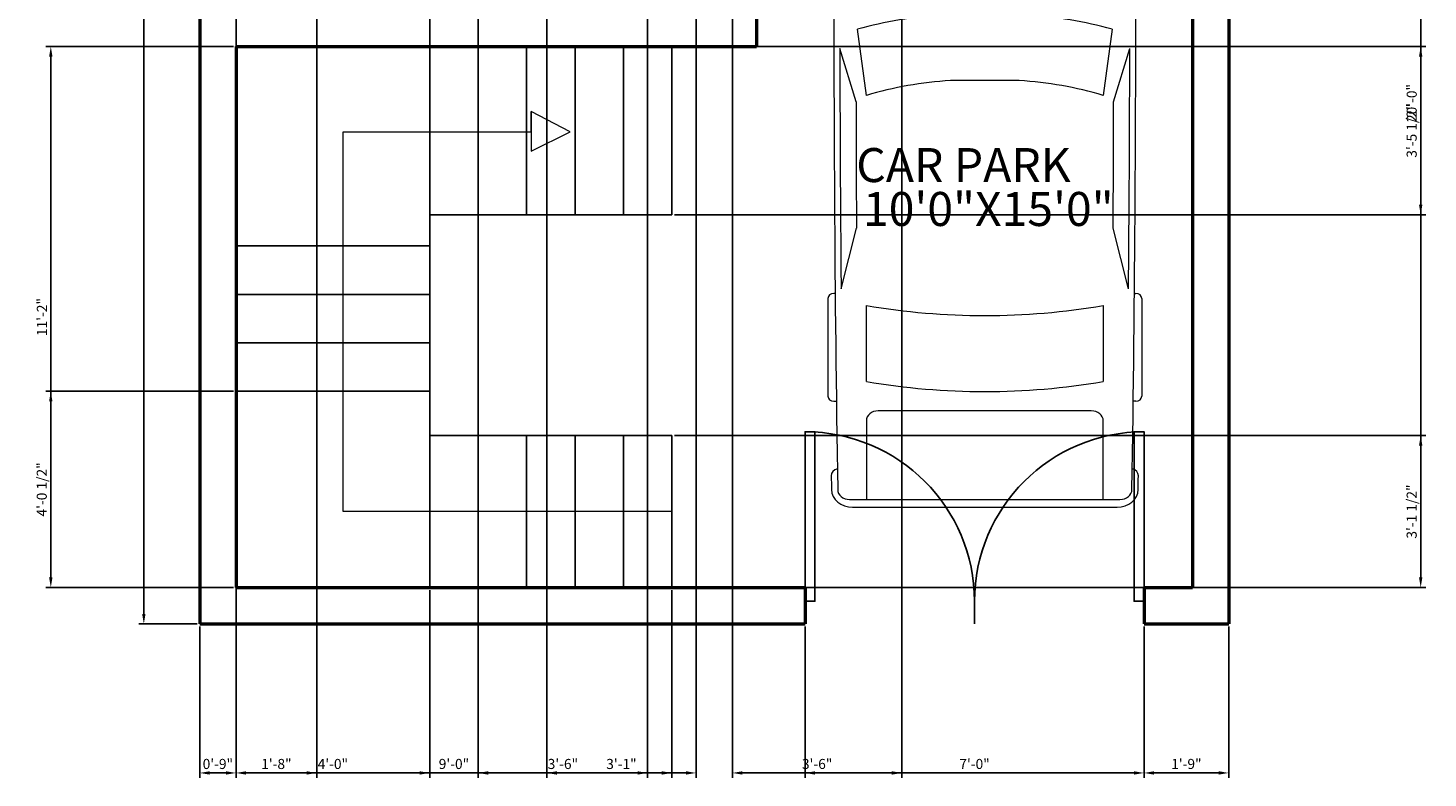
# Model space of a CAD drawing. Units: inches. Extents: x 758743 to 759108, y 3712801 to 3713581.
# Tile 1 of 4: x 758743 to 759090, y 3712801 to 3712987. Entities that reach past the tile are written whole.
import ezdxf

# ---------------------------------------------------------------- set-up
doc = ezdxf.new("R2010")
doc.units = ezdxf.units.IN
for name, color, linetype, lineweight in [('A-ANNO-DIMS', 2, 'Continuous', 18), ('A-ANNO-SYMB', 6, 'Continuous', 18), ('A-AREA-IDEN', 3, 'Continuous', 18), ('A-SITE-VEHI', 8, 'Continuous', 13), ('DOOR', 4, 'Continuous', 25), ('STAIRCASE', 6, 'Continuous', 25), ('WALL', 7, 'Continuous', 50)]:
    doc.layers.add(name, color=color, linetype=linetype, lineweight=lineweight)
doc.styles.get("Standard").update_dxf_attribs({"font": 'arial.ttf'})
doc.dimstyles.new('ISO-25', dxfattribs={"dimtxt": 2.5, "dimasz": 2.5, "dimexe": 1.25, "dimexo": 0.625, "dimtad": 1, "dimdec": 0, "dimlunit": 3, "dimtxsty": 'Standard', "dimcen": 2.5, "dimadec": 0, "dimazin": 0, "dimtfac": 1, "dimtdec": 0, "dimtmove": 0, "dimatfit": 3, "dimfxl": 1, "dimarcsym": 0})

# ---------------------------------------------------------------- blocks, each defined once
blk = doc.blocks.new('*U2')
for p, q in [((0, 0), (0, -100)), ((750, 0), (750, -100))]:
    blk.add_line(p, q)
blk.add_lwpolyline([(0, 0), (0, 750), (43.75, 750), (43.75, 0)], close=True)
blk.add_arc((0, 0), 750, 0, 90)
blk = doc.blocks.new('*U10')
for p, q in [((46.55, 38.89), (22.35, 38.89)), ((136.7, 38.89), (160.9, 38.89)), ((21.1, 37.41), (21.1, 36.83)), ((47.8, 37.39), (47.8, 37.41)), ((87.99, 31.87), (74.76, 35.92)), ((134.31, 35.6), (119.29, 31.78)), ((135.45, 37.07), (135.45, 37.41)), ((162.15, 37.41), (162.15, 36.77)), ((70.03, 31.54), (86.41, 29.35)), ((186.47, -33.5), (186.47, 33.5)), ((188.4, -32.76), (188.4, 32.76)), ((138.42, 29.35), (157.25, 29.35)), ((186.47, 29.35), (167.01, 29.35)), ((164.52, 26.39), (164.52, -26.39)), ((32.27, 11.63), (36.13, 17.17)), ((36.13, 17.17), (50.94, 17.17)), ((32.12, 9.51), (32.12, 11.15)), ((58.92, -10.77), (58.92, 10.77)), ((66.55, -10.53), (66.55, 10.53)), ((186.47, -10.53), (186.47, 10.53)), ((29.77, 9.51), (51.68, 9.51)), ((82.74, 8.5), (82.74, -8.5)), ((3.27, 6.13), (0.1, 0.41)), ((0, 0), (51.68, 0)), ((0.1, -0.41), (3.27, -6.13)), ((29.77, -9.51), (51.68, -9.51)), ((32.12, -9.51), (32.12, -11.15)), ((32.27, -11.63), (36.13, -17.17)), ((36.13, -17.17), (50.94, -17.17)), ((86.41, -29.35), (70.03, -31.54)), ((157.25, -29.35), (138.42, -29.35)), ((167.01, -29.35), (186.47, -29.35)), ((87.99, -31.87), (74.76, -35.92)), ((134.31, -35.6), (119.29, -31.78)), ((21.1, -37.41), (21.1, -36.83)), ((47.8, -37.39), (47.8, -37.41)), ((135.45, -37.07), (135.45, -37.41)), ((162.15, -37.41), (162.15, -36.77)), ((46.55, -38.89), (22.35, -38.89)), ((136.7, -38.89), (160.9, -38.89))]:
    blk.add_line(p, q)
for centre, major_axis, ratio, start_param, end_param in [((22.35, 37.41), (0, -1.48), 0.842304, 3.141593, 4.712389), ((46.55, 37.41), (0, 1.48), 0.842304, -1.570796, 0), ((136.7, 37.41), (0, -1.48), 0.842304, 3.141593, 4.712389), ((160.9, 37.41), (0, 1.48), 0.842304, -1.570796, 0), ((266.03, -27.52), (0, 313.31), 0.842304, 1.367076, 1.39176), ((41.19, -490.86), (0, 528.23), 0.842304, 0.00281, 0.075598), ((64.48, -10555.62), (0, 10593.03), 0.842304, -0.013397, 0.002797), ((64.48, -10555.62), (0, -10591.55), 0.842304, 3.133765, 3.140441), ((180.63, 35.84), (0, 2.22), 0.842304, -0.013017, 1.249894), ((64.48, -10556.36), (0, 10595.31), 0.842304, -0.013397, -0.013017), ((183.98, 33.5), (0, -2.96), 0.842304, 1.570796, 3.128196), ((183.98, 32.76), (0, -5.25), 0.842304, 1.570796, 3.128196), ((135.29, 5.39), (0, 81.77), 0.842304, 1.245306, 1.50788), ((95.79, -3666.35), (0, -3698.24), 0.842304, 3.134049, 3.144098), ((259.18, -27.52), (0, -305.3), 0.842304, 4.528606, 4.561838), ((37.47, -593.96), (0, -623.33), 0.842304, 3.096046, 3.200911), ((134.4, 5.39), (0, -89.78), 0.842304, 4.449482, 4.652344), ((149.6, 2.8), (0, -79.58), 0.842304, 4.372215, 4.640744), ((17.08, 0), (0, 147.02), 0.842304, 4.511394, 4.913384), ((35.91, 0), (0, 147.02), 0.842304, 4.511394, 4.913384), ((167.01, 26.39), (0, 2.96), 0.842304, 0, 1.570796), ((-204.49, 52.4), (0, -250.96), 0.842304, 1.385369, 1.434372), ((13.04, 17.01), (0, 27.42), 0.842304, 4.435146, 4.718221), ((14.2, 17.01), (0, 27.42), 0.842304, 4.435146, 4.718221), ((50.79, 13.34), (6.34, -0.36), 0.603834, -1.395552, 1.581315), ((32.75, 11.15), (0, 0.74), 0.842304, 0.879714, 1.570796), ((29.77, -46.66), (0, 56.17), 0.842304, 0, 0.590319), ((0.62, 0), (0, -0.74), 0.842304, 4.131459, 5.293319), ((29.77, 46.66), (0, 56.17), 0.842304, 2.551274, 3.141593), ((-204.49, -52.4), (0, 250.96), 0.842304, -1.434372, -1.385369), ((13.04, -17.01), (0, -27.42), 0.842304, 1.564964, 1.848039), ((14.2, -17.01), (0, -27.42), 0.842304, 1.564964, 1.848039), ((149.6, -2.8), (0, -79.58), 0.842304, -1.499151, -1.230623), ((32.75, -11.15), (0, -0.74), 0.842304, 4.712389, 5.403472), ((134.4, -5.39), (0, -89.78), 0.842304, -1.510751, -1.307889), ((135.29, -5.39), (0, -81.77), 0.842304, -1.50788, -1.245306), ((259.18, 27.52), (0, 305.3), 0.842304, 1.721348, 1.754579), ((167.01, -26.39), (0, -2.96), 0.842304, 4.712389, 6.283185), ((266.03, 27.52), (0, 313.31), 0.842304, 1.749832, 1.774517), ((37.47, 593.96), (0, -623.33), 0.842304, -0.059319, 0.045547), ((95.79, 3666.35), (0, -3698.24), 0.842304, -0.002505, 0.007544), ((183.98, -33.5), (0, 2.96), 0.842304, 3.15499, 4.712389), ((183.98, -32.76), (0, -5.25), 0.842304, 0.013397, 1.570796), ((41.19, 490.86), (0, -528.23), 0.842304, -0.075598, -0.00281), ((22.35, -37.41), (0, 1.48), 0.842304, 1.570796, 3.141593), ((64.48, 10555.62), (0, 10593.03), 0.842304, 3.138796, 3.15499), ((46.55, -37.41), (0, -1.48), 0.842304, 0, 1.570796), ((64.48, 10555.62), (0, -10591.55), 0.842304, 0.001152, 0.007828), ((136.7, -37.41), (0, -1.48), 0.842304, -1.570796, 0), ((160.9, -37.41), (0, 1.48), 0.842304, 3.141593, 4.712389), ((180.63, -35.84), (0, -2.22), 0.842304, -1.249894, 0.013017), ((64.48, 10556.36), (0, 10595.31), 0.842304, 3.15461, 3.15499)]:
    blk.add_ellipse(centre, major_axis=major_axis, ratio=ratio, start_param=start_param, end_param=end_param)
at = {"extrusion": (0, 0, -1)}
blk.add_ellipse((50.79, -13.34), major_axis=(6.34, 0.36), ratio=0.603834, start_param=-1.395552, end_param=1.581315, dxfattribs=at)
blk = doc.blocks.new('*D13')
at = {"layer": 'A-ANNO-DIMS', "color": 0, "lineweight": -2, "transparency": 16777216}
for p, q in [((758785.26, 3713540.49), (758770.79, 3713540.49)), ((758772.04, 3713537.99), (758772.04, 3712841.99)), ((758785.26, 3712839.49), (758770.79, 3712839.49))]:
    blk.add_line(p, q, dxfattribs=at)
at = {"layer": 'A-ANNO-DIMS', "color": 0, "transparency": 16777216}
for points in [[(758771.62, 3713537.99), (758772.46, 3713537.99), (758772.04, 3713540.49)], [(758771.62, 3712841.99), (758772.46, 3712841.99), (758772.04, 3712839.49)]]:
    blk.add_solid(points, dxfattribs=at)
at = {"layer": 'Defpoints', "color": 0, "transparency": 16777216}
for p in [(758785.89, 3713540.49), (758772.04, 3712839.49), (758785.89, 3712839.49)]:
    blk.add_point(p, dxfattribs=at)
at = {"layer": 'A-ANNO-DIMS', "color": 0, "transparency": 16777216, "insert": (758770.14, 3713189.99), "char_height": 2.5, "attachment_point": 5, "rotation": 90}
blk.add_mtext('58\'-5"', dxfattribs=at)
blk = doc.blocks.new('*D42')
at = {"layer": 'A-ANNO-DIMS', "color": 0, "lineweight": -2, "transparency": 16777216}
for p, q in [((758935.89, 3712838.87), (758935.89, 3712801.34)), ((759019.89, 3712838.87), (759019.89, 3712801.34)), ((758938.39, 3712802.59), (759017.39, 3712802.59))]:
    blk.add_line(p, q, dxfattribs=at)
at = {"layer": 'A-ANNO-DIMS', "color": 0, "transparency": 16777216}
for points in [[(758938.39, 3712803.01), (758938.39, 3712802.17), (758935.89, 3712802.59)], [(759017.39, 3712803.01), (759017.39, 3712802.17), (759019.89, 3712802.59)]]:
    blk.add_solid(points, dxfattribs=at)
at = {"layer": 'Defpoints', "color": 0, "transparency": 16777216}
for p in [(758935.89, 3712839.49), (759019.89, 3712839.49), (759019.89, 3712802.59)]:
    blk.add_point(p, dxfattribs=at)
at = {"layer": 'A-ANNO-DIMS', "color": 0, "transparency": 16777216, "insert": (758977.89, 3712804.49), "char_height": 2.5, "attachment_point": 5}
blk.add_mtext('7\'-0"', dxfattribs=at)
blk = doc.blocks.new('*D43')
at = {"layer": 'A-ANNO-DIMS', "color": 0, "lineweight": -2, "transparency": 16777216}
for p, q in [((759019.89, 3712838.87), (759019.89, 3712801.34)), ((759040.89, 3712838.87), (759040.89, 3712801.34)), ((759022.39, 3712802.59), (759038.39, 3712802.59))]:
    blk.add_line(p, q, dxfattribs=at)
at = {"layer": 'A-ANNO-DIMS', "color": 0, "transparency": 16777216}
for points in [[(759022.39, 3712803.01), (759022.39, 3712802.17), (759019.89, 3712802.59)], [(759038.39, 3712803.01), (759038.39, 3712802.17), (759040.89, 3712802.59)]]:
    blk.add_solid(points, dxfattribs=at)
at = {"layer": 'Defpoints', "color": 0, "transparency": 16777216}
for p in [(759019.89, 3712839.49), (759040.89, 3712839.49), (759040.89, 3712802.59)]:
    blk.add_point(p, dxfattribs=at)
at = {"layer": 'A-ANNO-DIMS', "color": 0, "transparency": 16777216, "insert": (759030.39, 3712804.49), "char_height": 2.5, "attachment_point": 5}
blk.add_mtext('1\'-9"', dxfattribs=at)
blk = doc.blocks.new('*D44')
at = {"layer": 'A-ANNO-DIMS', "color": 0, "lineweight": -2, "transparency": 16777216}
for p, q in [((758794.89, 3712847.87), (758794.89, 3712801.34)), ((758902.89, 3712847.87), (758902.89, 3712801.34)), ((758797.39, 3712802.59), (758900.39, 3712802.59))]:
    blk.add_line(p, q, dxfattribs=at)
at = {"layer": 'A-ANNO-DIMS', "color": 0, "transparency": 16777216}
for points in [[(758797.39, 3712803.01), (758797.39, 3712802.17), (758794.89, 3712802.59)], [(758900.39, 3712803.01), (758900.39, 3712802.17), (758902.89, 3712802.59)]]:
    blk.add_solid(points, dxfattribs=at)
at = {"layer": 'Defpoints', "color": 0, "transparency": 16777216}
for p in [(758794.89, 3712848.49), (758902.89, 3712848.49), (758902.89, 3712802.59)]:
    blk.add_point(p, dxfattribs=at)
at = {"layer": 'A-ANNO-DIMS', "color": 0, "transparency": 16777216, "insert": (758848.89, 3712804.49), "char_height": 2.5, "attachment_point": 5}
blk.add_mtext('9\'-0"', dxfattribs=at)
blk = doc.blocks.new('*D45')
at = {"layer": 'A-ANNO-DIMS', "color": 0, "lineweight": -2, "transparency": 16777216}
for p, q in [((758794.26, 3712982.49), (758747.74, 3712982.49)), ((758748.99, 3712850.99), (758748.99, 3712979.99)), ((758794.26, 3712848.49), (758747.74, 3712848.49))]:
    blk.add_line(p, q, dxfattribs=at)
at = {"layer": 'A-ANNO-DIMS', "color": 0, "transparency": 16777216}
for points in [[(758748.57, 3712979.99), (758749.4, 3712979.99), (758748.99, 3712982.49)], [(758748.57, 3712850.99), (758749.4, 3712850.99), (758748.99, 3712848.49)]]:
    blk.add_solid(points, dxfattribs=at)
at = {"layer": 'Defpoints', "color": 0, "transparency": 16777216}
for p in [(758748.99, 3712982.49), (758794.89, 3712982.49), (758794.89, 3712848.49)]:
    blk.add_point(p, dxfattribs=at)
at = {"layer": 'A-ANNO-DIMS', "color": 0, "transparency": 16777216, "insert": (758747.11, 3712915.49), "char_height": 2.5, "attachment_point": 5, "rotation": 90}
blk.add_mtext('11\'-2"', dxfattribs=at)
blk = doc.blocks.new('*D46')
at = {"layer": 'A-ANNO-DIMS', "color": 0, "lineweight": -2, "transparency": 16777216}
for p, q in [((758842.89, 3712849.12), (758842.89, 3713578.64)), ((758854.89, 3712849.12), (758854.89, 3713578.64)), ((758845.39, 3713577.39), (758852.39, 3713577.39))]:
    blk.add_line(p, q, dxfattribs=at)
at = {"layer": 'A-ANNO-DIMS', "color": 0, "transparency": 16777216}
for points in [[(758845.39, 3713577.81), (758845.39, 3713576.97), (758842.89, 3713577.39)], [(758852.39, 3713577.81), (758852.39, 3713576.97), (758854.89, 3713577.39)]]:
    blk.add_solid(points, dxfattribs=at)
at = {"layer": 'Defpoints', "color": 0, "transparency": 16777216}
for p in [(758854.89, 3713577.39), (758842.89, 3712848.49), (758854.89, 3712848.49)]:
    blk.add_point(p, dxfattribs=at)
at = {"layer": 'A-ANNO-DIMS', "color": 0, "transparency": 16777216, "insert": (758848.89, 3713579.29), "char_height": 2.5, "attachment_point": 5}
blk.add_mtext('1\'-0"', dxfattribs=at)
blk = doc.blocks.new('*D47')
at = {"layer": 'A-ANNO-DIMS', "color": 0, "lineweight": -2, "transparency": 16777216}
for p, q in [((758794.89, 3712847.87), (758794.89, 3712801.34)), ((758785.89, 3712838.87), (758785.89, 3712801.34)), ((758788.39, 3712802.59), (758792.39, 3712802.59))]:
    blk.add_line(p, q, dxfattribs=at)
at = {"layer": 'A-ANNO-DIMS', "color": 0, "transparency": 16777216}
for points in [[(758788.39, 3712803.01), (758788.39, 3712802.17), (758785.89, 3712802.59)], [(758792.39, 3712803.01), (758792.39, 3712802.17), (758794.89, 3712802.59)]]:
    blk.add_solid(points, dxfattribs=at)
at = {"layer": 'Defpoints', "color": 0, "transparency": 16777216}
for p in [(758794.89, 3712848.49), (758785.89, 3712839.49), (758794.89, 3712802.59)]:
    blk.add_point(p, dxfattribs=at)
at = {"layer": 'A-ANNO-DIMS', "color": 0, "transparency": 16777216, "insert": (758790.39, 3712804.49), "char_height": 2.5, "attachment_point": 5}
blk.add_mtext('0\'-9"', dxfattribs=at)
blk = doc.blocks.new('*D48')
at = {"layer": 'A-ANNO-DIMS', "color": 0, "lineweight": -2, "transparency": 16777216}
for p, q in [((758794.89, 3712847.87), (758794.89, 3712801.34)), ((758842.89, 3712847.87), (758842.89, 3712801.34)), ((758797.39, 3712802.59), (758840.39, 3712802.59))]:
    blk.add_line(p, q, dxfattribs=at)
at = {"layer": 'A-ANNO-DIMS', "color": 0, "transparency": 16777216}
for points in [[(758797.39, 3712803.01), (758797.39, 3712802.17), (758794.89, 3712802.59)], [(758840.39, 3712803.01), (758840.39, 3712802.17), (758842.89, 3712802.59)]]:
    blk.add_solid(points, dxfattribs=at)
at = {"layer": 'Defpoints', "color": 0, "transparency": 16777216}
for p in [(758794.89, 3712848.49), (758842.89, 3712848.49), (758842.89, 3712802.59)]:
    blk.add_point(p, dxfattribs=at)
at = {"layer": 'A-ANNO-DIMS', "color": 0, "transparency": 16777216, "insert": (758818.89, 3712804.49), "char_height": 2.5, "attachment_point": 5}
blk.add_mtext('4\'-0"', dxfattribs=at)
blk = doc.blocks.new('*D50')
at = {"layer": 'A-ANNO-DIMS', "color": 0, "lineweight": -2, "transparency": 16777216}
for p, q in [((758794.89, 3713312.87), (758794.89, 3712801.34)), ((758814.89, 3713312.87), (758814.89, 3712801.34)), ((758797.39, 3712802.59), (758812.39, 3712802.59))]:
    blk.add_line(p, q, dxfattribs=at)
at = {"layer": 'A-ANNO-DIMS', "color": 0, "transparency": 16777216}
for points in [[(758797.39, 3712803.01), (758797.39, 3712802.17), (758794.89, 3712802.59)], [(758812.39, 3712803.01), (758812.39, 3712802.17), (758814.89, 3712802.59)]]:
    blk.add_solid(points, dxfattribs=at)
at = {"layer": 'Defpoints', "color": 0, "transparency": 16777216}
for p in [(758794.89, 3713313.49), (758814.89, 3713313.49), (758814.89, 3712802.59)]:
    blk.add_point(p, dxfattribs=at)
at = {"layer": 'A-ANNO-DIMS', "color": 0, "transparency": 16777216, "insert": (758804.89, 3712804.49), "char_height": 2.5, "attachment_point": 5}
blk.add_mtext('1\'-8"', dxfattribs=at)
blk = doc.blocks.new('*D52')
at = {"layer": 'A-ANNO-DIMS', "color": 0, "lineweight": -2, "transparency": 16777216}
for p, q in [((758871.89, 3713158.87), (758871.89, 3712801.34)), ((758908.89, 3713158.87), (758908.89, 3712801.34)), ((758874.39, 3712802.59), (758906.39, 3712802.59))]:
    blk.add_line(p, q, dxfattribs=at)
at = {"layer": 'A-ANNO-DIMS', "color": 0, "transparency": 16777216}
for points in [[(758874.39, 3712803.01), (758874.39, 3712802.17), (758871.89, 3712802.59)], [(758906.39, 3712803.01), (758906.39, 3712802.17), (758908.89, 3712802.59)]]:
    blk.add_solid(points, dxfattribs=at)
at = {"layer": 'Defpoints', "color": 0, "transparency": 16777216}
for p in [(758871.89, 3713159.49), (758908.89, 3713159.49), (758908.89, 3712802.59)]:
    blk.add_point(p, dxfattribs=at)
at = {"layer": 'A-ANNO-DIMS', "color": 0, "transparency": 16777216, "insert": (758890.39, 3712804.49), "char_height": 2.5, "attachment_point": 5}
blk.add_mtext('3\'-1"', dxfattribs=at)
blk = doc.blocks.new('*D54')
at = {"layer": 'A-ANNO-DIMS', "color": 0, "lineweight": -2, "transparency": 16777216}
for p, q in [((758854.89, 3713405.87), (758854.89, 3712801.34)), ((758896.89, 3713405.87), (758896.89, 3712801.34)), ((758857.39, 3712802.59), (758894.39, 3712802.59))]:
    blk.add_line(p, q, dxfattribs=at)
at = {"layer": 'A-ANNO-DIMS', "color": 0, "transparency": 16777216}
for points in [[(758857.39, 3712803.01), (758857.39, 3712802.17), (758854.89, 3712802.59)], [(758894.39, 3712803.01), (758894.39, 3712802.17), (758896.89, 3712802.59)]]:
    blk.add_solid(points, dxfattribs=at)
at = {"layer": 'Defpoints', "color": 0, "transparency": 16777216}
for p in [(758854.89, 3713406.49), (758896.89, 3713406.49), (758896.89, 3712802.59)]:
    blk.add_point(p, dxfattribs=at)
at = {"layer": 'A-ANNO-DIMS', "color": 0, "transparency": 16777216, "insert": (758875.89, 3712804.49), "char_height": 2.5, "attachment_point": 5}
blk.add_mtext('3\'-6"', dxfattribs=at)
blk = doc.blocks.new('*D55')
at = {"layer": 'A-ANNO-DIMS', "color": 0, "lineweight": -2, "transparency": 16777216}
for p, q in [((759032.51, 3713088.49), (759089.7, 3713088.49)), ((759088.45, 3712850.99), (759088.45, 3713085.99)), ((759032.51, 3712848.49), (759089.7, 3712848.49))]:
    blk.add_line(p, q, dxfattribs=at)
at = {"layer": 'A-ANNO-DIMS', "color": 0, "transparency": 16777216}
for points in [[(759088.04, 3713085.99), (759088.87, 3713085.99), (759088.45, 3713088.49)], [(759088.04, 3712850.99), (759088.87, 3712850.99), (759088.45, 3712848.49)]]:
    blk.add_solid(points, dxfattribs=at)
at = {"layer": 'Defpoints', "color": 0, "transparency": 16777216}
for p in [(759031.89, 3713088.49), (759088.45, 3713088.49), (759031.89, 3712848.49)]:
    blk.add_point(p, dxfattribs=at)
at = {"layer": 'A-ANNO-DIMS', "color": 0, "transparency": 16777216, "insert": (759086.55, 3712968.49), "char_height": 2.5, "attachment_point": 5, "rotation": 90}
blk.add_mtext('20\'-0"', dxfattribs=at)
blk = doc.blocks.new('*D56')
at = {"layer": 'A-ANNO-DIMS', "color": 0, "lineweight": -2, "transparency": 16777216}
for p, q in [((758903.51, 3712886.14), (759089.7, 3712886.14)), ((759088.45, 3712850.99), (759088.45, 3712883.64)), ((758903.51, 3712848.49), (759089.7, 3712848.49))]:
    blk.add_line(p, q, dxfattribs=at)
at = {"layer": 'A-ANNO-DIMS', "color": 0, "transparency": 16777216}
for points in [[(759088.04, 3712883.64), (759088.87, 3712883.64), (759088.45, 3712886.14)], [(759088.04, 3712850.99), (759088.87, 3712850.99), (759088.45, 3712848.49)]]:
    blk.add_solid(points, dxfattribs=at)
at = {"layer": 'Defpoints', "color": 0, "transparency": 16777216}
for p in [(758902.89, 3712886.14), (759088.45, 3712886.14), (758902.89, 3712848.49)]:
    blk.add_point(p, dxfattribs=at)
at = {"layer": 'A-ANNO-DIMS', "color": 0, "transparency": 16777216, "insert": (759086.54, 3712867.32), "char_height": 2.5, "attachment_point": 5, "rotation": 90}
blk.add_mtext('3\'-1 1/2"', dxfattribs=at)
blk = doc.blocks.new('*D57')
at = {"layer": 'A-ANNO-DIMS', "color": 0, "lineweight": -2, "transparency": 16777216}
for p, q in [((758903.51, 3712982.49), (759089.7, 3712982.49)), ((759088.45, 3712943.32), (759088.45, 3712979.99)), ((758903.51, 3712940.82), (759089.7, 3712940.82))]:
    blk.add_line(p, q, dxfattribs=at)
at = {"layer": 'A-ANNO-DIMS', "color": 0, "transparency": 16777216}
for points in [[(759088.04, 3712979.99), (759088.87, 3712979.99), (759088.45, 3712982.49)], [(759088.04, 3712943.32), (759088.87, 3712943.32), (759088.45, 3712940.82)]]:
    blk.add_solid(points, dxfattribs=at)
at = {"layer": 'Defpoints', "color": 0, "transparency": 16777216}
for p in [(758902.89, 3712982.49), (759088.45, 3712982.49), (758902.89, 3712940.82)]:
    blk.add_point(p, dxfattribs=at)
at = {"layer": 'A-ANNO-DIMS', "color": 0, "transparency": 16777216, "insert": (759086.54, 3712961.66), "char_height": 2.5, "attachment_point": 5, "rotation": 90}
blk.add_mtext('3\'-5 1/2"', dxfattribs=at)
blk = doc.blocks.new('*D58')
at = {"layer": 'A-ANNO-DIMS', "color": 0, "lineweight": -2, "transparency": 16777216}
for p, q in [((758794.26, 3712897.11), (758747.74, 3712897.11)), ((758748.99, 3712850.99), (758748.99, 3712894.61)), ((758794.26, 3712848.49), (758747.74, 3712848.49))]:
    blk.add_line(p, q, dxfattribs=at)
at = {"layer": 'A-ANNO-DIMS', "color": 0, "transparency": 16777216}
for points in [[(758748.57, 3712894.61), (758749.4, 3712894.61), (758748.99, 3712897.11)], [(758748.57, 3712850.99), (758749.4, 3712850.99), (758748.99, 3712848.49)]]:
    blk.add_solid(points, dxfattribs=at)
at = {"layer": 'Defpoints', "color": 0, "transparency": 16777216}
for p in [(758748.99, 3712897.11), (758794.89, 3712897.11), (758794.89, 3712848.49)]:
    blk.add_point(p, dxfattribs=at)
at = {"layer": 'A-ANNO-DIMS', "color": 0, "transparency": 16777216, "insert": (758747.07, 3712872.8), "char_height": 2.5, "attachment_point": 5, "rotation": 90}
blk.add_mtext('4\'-0 1/2"', dxfattribs=at)
blk = doc.blocks.new('*D59')
at = {"layer": 'A-ANNO-DIMS', "color": 0, "lineweight": -2, "transparency": 16777216}
for p, q in [((758917.89, 3713405.87), (758917.89, 3712801.34)), ((758959.89, 3713405.87), (758959.89, 3712801.34)), ((758920.39, 3712802.59), (758957.39, 3712802.59))]:
    blk.add_line(p, q, dxfattribs=at)
at = {"layer": 'A-ANNO-DIMS', "color": 0, "transparency": 16777216}
for points in [[(758920.39, 3712803.01), (758920.39, 3712802.17), (758917.89, 3712802.59)], [(758957.39, 3712803.01), (758957.39, 3712802.17), (758959.89, 3712802.59)]]:
    blk.add_solid(points, dxfattribs=at)
at = {"layer": 'Defpoints', "color": 0, "transparency": 16777216}
for p in [(758917.89, 3713406.49), (758959.89, 3713406.49), (758959.89, 3712802.59)]:
    blk.add_point(p, dxfattribs=at)
at = {"layer": 'A-ANNO-DIMS', "color": 0, "transparency": 16777216, "insert": (758938.89, 3712804.49), "char_height": 2.5, "attachment_point": 5}
blk.add_mtext('3\'-6"', dxfattribs=at)

msp = doc.modelspace()

# ---------------------------------------------------------------- linework, layer by layer
at = {"layer": 'A-ANNO-SYMB'}
for p, q in [((758868, 3712961.39), (758868, 3712966.38)), ((758868, 3712966.38), (758868, 3712956.59)), ((758877.68, 3712961.39), (758868, 3712966.38)), ((758821.42, 3712867.32), (758821.42, 3712961.39)), ((758821.42, 3712961.39), (758868, 3712961.39)), ((758868, 3712956.59), (758877.68, 3712961.39)), ((758902.89, 3712867.32), (758821.42, 3712867.32))]:
    msp.add_line(p, q, dxfattribs=at)
at = {"layer": 'STAIRCASE'}
for p, q in [((758842.89, 3712982.49), (758842.89, 3712848.49)), ((758854.89, 3712982.49), (758854.89, 3712940.82)), ((758866.89, 3712982.49), (758866.89, 3712940.82)), ((758878.89, 3712982.49), (758878.89, 3712940.82)), ((758890.89, 3712982.49), (758890.89, 3712940.82)), ((758902.89, 3712982.49), (758902.89, 3712940.82)), ((758842.89, 3712886.14), (758842.89, 3712940.82)), ((758842.89, 3712940.82), (758902.89, 3712940.82)), ((758842.89, 3712933.11), (758794.89, 3712933.11)), ((758842.89, 3712921.11), (758794.89, 3712921.11)), ((758842.89, 3712909.11), (758794.89, 3712909.11)), ((758842.89, 3712897.11), (758794.89, 3712897.11)), ((758902.89, 3712886.14), (758842.89, 3712886.14)), ((758854.89, 3712886.14), (758854.89, 3712848.49)), ((758866.89, 3712886.14), (758866.89, 3712848.49)), ((758878.89, 3712886.14), (758878.89, 3712848.49)), ((758890.89, 3712886.14), (758890.89, 3712848.49)), ((758902.89, 3712886.14), (758902.89, 3712848.49))]:
    msp.add_line(p, q, dxfattribs=at)
at = {"layer": 'WALL'}
for p, q in [((758785.89, 3713540.49), (758785.89, 3712839.49)), ((759040.89, 3713540.49), (759040.89, 3712839.49)), ((759031.89, 3713406.49), (759031.89, 3712848.49)), ((758923.89, 3713097.49), (758923.89, 3712982.49)), ((758794.89, 3712982.49), (758923.89, 3712982.49)), ((758794.89, 3712982.49), (758794.89, 3712848.49)), ((758794.89, 3712848.49), (758935.89, 3712848.49)), ((758923.89, 3712848.49), (758935.89, 3712848.49)), ((758935.89, 3712848.49), (758935.89, 3712839.49)), ((759019.89, 3712848.49), (759019.89, 3712839.49)), ((759019.89, 3712848.49), (759031.89, 3712848.49)), ((758785.89, 3712839.49), (758935.89, 3712839.49)), ((759019.89, 3712839.49), (759040.89, 3712839.49))]:
    msp.add_line(p, q, dxfattribs=at)

# ---------------------------------------------------------------- block references
at = {"layer": 'A-SITE-VEHI', "rotation": 270}
msp.add_blockref('*U10', (758980.44, 3713056.78), dxfattribs=at)
at = {"layer": 'DOOR', "yscale": 0.0559999999999739, "zscale": 0.0559999999999739}
for p, xscale in [((758935.89, 3712845.09), 0.0559999999999739), ((759019.89, 3712845.09), -0.0559999999999739)]:
    msp.add_blockref('*U2', p, dxfattribs=dict(at, xscale=xscale))

# ---------------------------------------------------------------- texts
at = {"layer": 'A-AREA-IDEN'}
for s, height, p in [('CAR PARK', 8.421, (758948.58, 3712948.91)), ('10\'0"X15\'0"', 8.4209, (758950.25, 3712938.04))]:
    msp.add_text(s, height=height, dxfattribs=at).set_placement(p)

# ---------------------------------------------------------------- dimensions: what is measured, and where the dimension line sits
at = {"layer": 'A-ANNO-DIMS'}
for base, p1, p2, picture, middle in [((758854.89, 3713577.39), (758842.89, 3712848.49), (758854.89, 3712848.49), '*D46', (758848.89, 3713579.29)), ((758896.89, 3712802.59), (758854.89, 3713406.49), (758896.89, 3713406.49), '*D54', (758875.89, 3712804.49)), ((758959.89, 3712802.59), (758917.89, 3713406.49), (758959.89, 3713406.49), '*D59', (758938.89, 3712804.49)), ((758814.89, 3712802.59), (758794.89, 3713313.49), (758814.89, 3713313.49), '*D50', (758804.89, 3712804.49)), ((758908.89, 3712802.59), (758871.89, 3713159.49), (758908.89, 3713159.49), '*D52', (758890.39, 3712804.49)), ((758794.89, 3712802.59), (758785.89, 3712839.49), (758794.89, 3712848.49), '*D47', (758790.39, 3712804.49)), ((758902.89, 3712802.59), (758794.89, 3712848.49), (758902.89, 3712848.49), '*D44', (758848.89, 3712804.49)), ((758842.89, 3712802.59), (758794.89, 3712848.49), (758842.89, 3712848.49), '*D48', (758818.89, 3712804.49)), ((759019.89, 3712802.59), (758935.89, 3712839.49), (759019.89, 3712839.49), '*D42', (758977.89, 3712804.49)), ((759040.89, 3712802.59), (759019.89, 3712839.49), (759040.89, 3712839.49), '*D43', (759030.39, 3712804.49))]:
    dim = msp.add_linear_dim(base=base, p1=p1, p2=p2, dimstyle='ISO-25', override={"dimdec": 1, "dimlfac": 1, "dimrnd": 0, "dimzin": 1, "dimdsep": 46, "dimlunit": 4, "dimfrac": 2}, dxfattribs=at)
    dim.commit()
    dim.dimension.update_dxf_attribs({"geometry": picture, "text_midpoint": middle})
for base, p1, p2, override, picture, middle in [((758772.04, 3712839.49), (758785.89, 3713540.49), (758785.89, 3712839.49), {"dimclrd": 0, "dimclre": 0, "dimclrt": 0}, '*D13', (758770.14, 3713189.99)), ((759088.45, 3713088.49), (759031.89, 3712848.49), (759031.89, 3713088.49), {"dimdec": 1, "dimlfac": 1, "dimrnd": 0, "dimzin": 1, "dimdsep": 46, "dimlunit": 4, "dimfrac": 2}, '*D55', (759086.55, 3712968.49)), ((758748.99, 3712982.49), (758794.89, 3712848.49), (758794.89, 3712982.49), {"dimdec": 1, "dimlfac": 1, "dimrnd": 0, "dimzin": 1, "dimdsep": 46, "dimlunit": 4, "dimfrac": 2}, '*D45', (758747.11, 3712915.49)), ((759088.45, 3712982.49), (758902.89, 3712940.82), (758902.89, 3712982.49), {"dimdec": 1, "dimlfac": 1, "dimrnd": 0, "dimzin": 1, "dimdsep": 46, "dimlunit": 4, "dimfrac": 2}, '*D57', (759086.54, 3712961.66)), ((758748.99, 3712897.11), (758794.89, 3712848.49), (758794.89, 3712897.11), {"dimdec": 1, "dimlfac": 1, "dimrnd": 0, "dimzin": 1, "dimdsep": 46, "dimlunit": 4, "dimfrac": 2}, '*D58', (758747.07, 3712872.8)), ((759088.4539, 3712886.145), (758902.8852, 3712848.4916), (758902.8852, 3712886.145), {"dimdec": 1, "dimlfac": 1, "dimrnd": 0, "dimzin": 1, "dimdsep": 46, "dimlunit": 4, "dimfrac": 2}, '*D56', (759086.5354, 3712867.3183))]:
    dim = msp.add_linear_dim(base=base, p1=p1, p2=p2, angle=90, dimstyle='ISO-25', override=override, dxfattribs=at)
    dim.commit()
    dim.dimension.update_dxf_attribs({"geometry": picture, "text_midpoint": middle})

doc.saveas('drawing.dxf')
